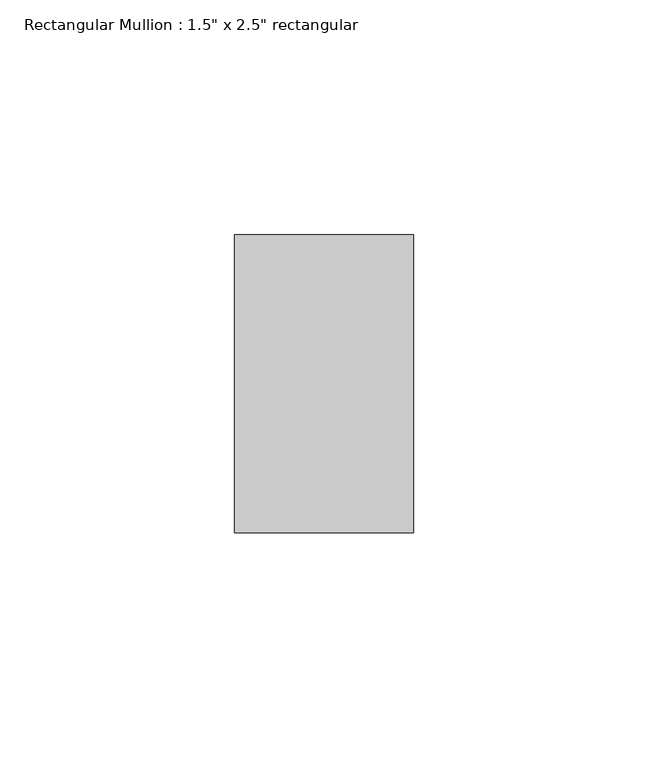
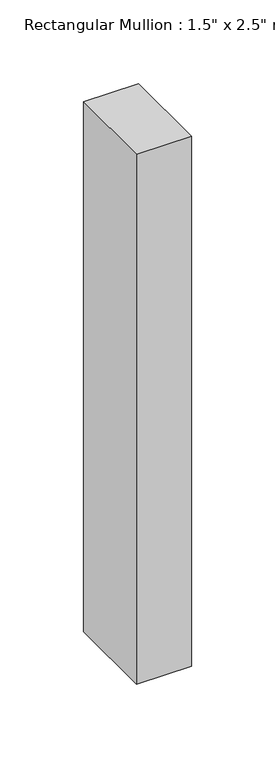
"""IFC4 building model written with IfcOpenShell, lengths in millimetres: member geometry."""

from ifc_helpers import new_model, si_unit, frame, origin, place, context, project, spatial, polyline, outline, extrude, source, transform, mapped, element, save


def member_eea045b6(model_context):
    return source(origin(), model_context, "Body", "SweptSolid", [
        extrude(outline(polyline([(19.05, 31.75), (19.05, -31.75), (-19.05, -31.75), (-19.05, 31.75), (19.05, 31.75)])), frame((0.0, 0.0, -387.35), z_axis=(0.0, 0.0, 1.0), x_axis=(1.0, 0.0, 0.0)), (0.0, 0.0, 1.0), 387.35),
    ])


if __name__ == "__main__":
    model = new_model("IFC4")
    model_context = context("Model", 3, world=origin())
    ifc_project = project(units=[si_unit("LENGTHUNIT", "METRE", prefix="MILLI")], contexts=[model_context])
    site = spatial("IfcSite", under=ifc_project)
    building = spatial("IfcBuilding", under=site)
    placement = place(None, origin())
    member_shape = member_eea045b6(model_context)
    element("IfcMember", 1, ObjectType="Rectangular Mullion : 1.5\" x 2.5\" rectangular", at=placement, inside=building, context=model_context, shape_type="MappedRepresentation", body=[
        mapped(member_shape, transform((0.0, 0.0, 0.0), x_axis=(1.0, 0.0, 0.0), y_axis=(0.0, 1.0, 0.0), z_axis=(0.0, 0.0, 1.0))),
    ])
    save(model, "model.ifc")

# Revit data of these elements
# Type "Rectangular Mullion : 1.5\" x 2.5\" rectangular"
#   built-in parameter 1007304 = 0.208333 (stored number, unit not read)
#   built-in parameter 1007301 = 0.0625 (stored number, unit not read)
#   built-in parameter 1007300 = 0.0625 (stored number, unit not read)
# Element 1 (IfcMember, "Rectangular Mullion : 1.5\" x 2.5\" rectangular")
#   Materials on its faces: "Aluminum"
# Materials
#   "Aluminum": class "Metal", colour RGB 247 247 247, transparency 0, Description = "Aluminum 6061", Cost = 0
